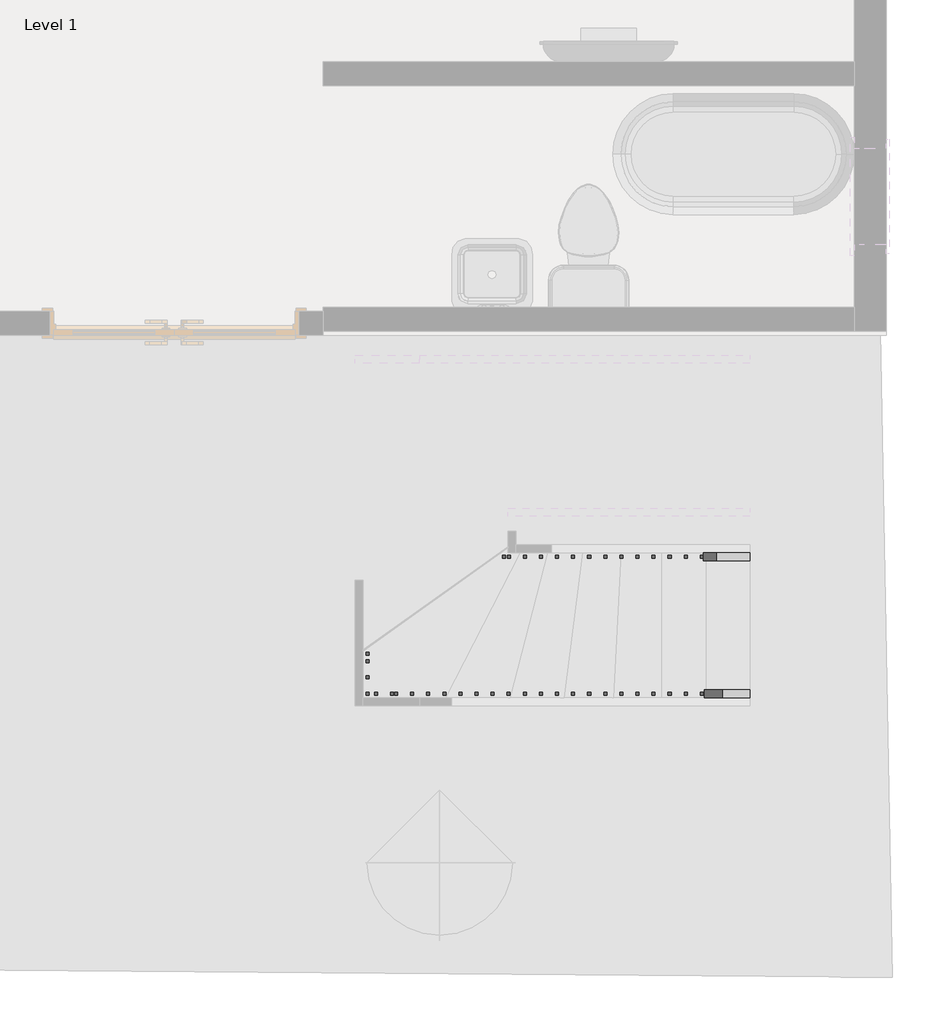
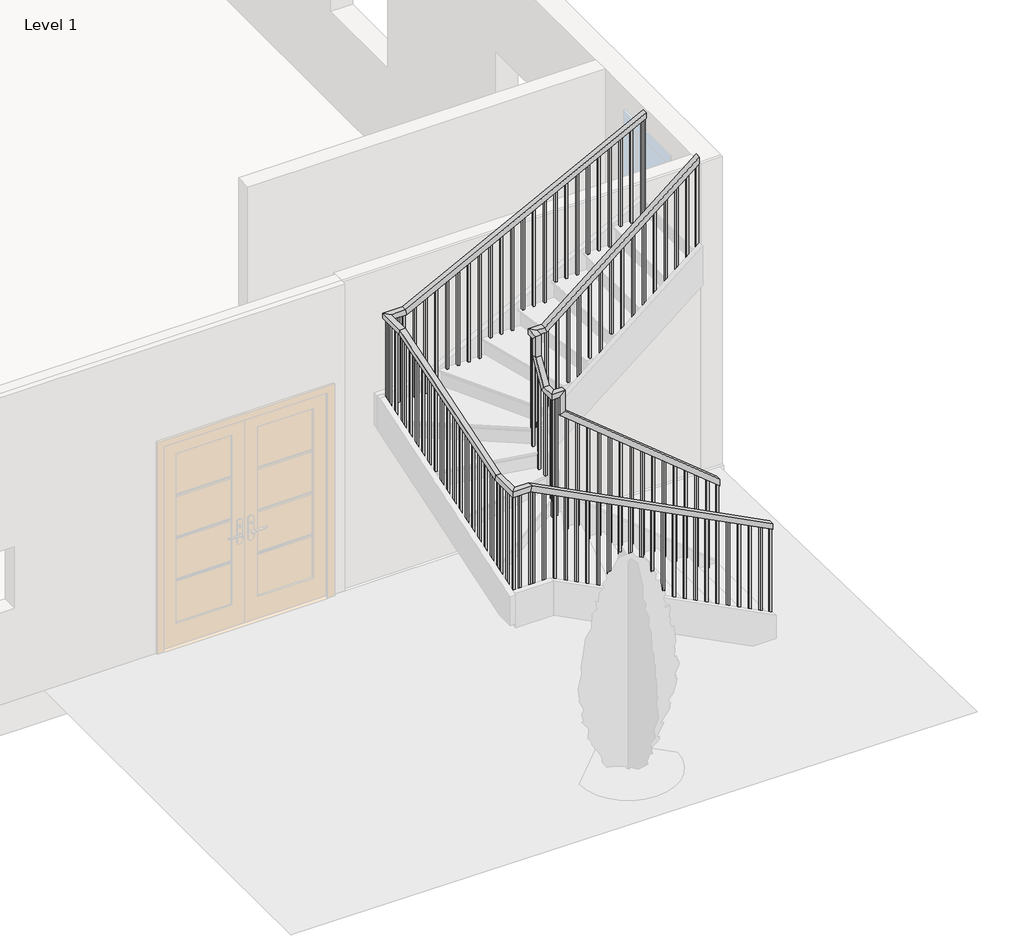
# One storey, part 2 of 3: 2 railings.
"""IFC4 building model written with IfcOpenShell, lengths in millimetres."""

from ifc_helpers import new_model, si_unit, frame, origin, place, context, project, spatial, polyline, outline, extrude, faceted_brep, element, save

model = new_model("IFC4")

# Units and contexts
model_context = context("Model", 3, world=origin())
ifc_project = project(units=[si_unit("LENGTHUNIT", "METRE", prefix="MILLI")], contexts=[model_context])

# Site, building, storey
site = spatial("IfcSite", under=ifc_project)
building = spatial("IfcBuilding", under=site)
storey = spatial("IfcBuildingStorey", under=building, Name="Level 1", Elevation=0.0)

# Railings
placement = place(None, origin())
element("IfcRailing", 1, ObjectType="Handrail - Rectangular", at=placement, inside=storey, context=model_context, shape_type="SolidModel", body=[
    faceted_brep([(-3425.4930658, -1530.446371, 1025.2529681), (-3425.4930658, -1530.446371, 959.7067088), (-3425.4930658, -1479.646371, 959.7067088), (-3425.4930658, -1479.646371, 1025.2529681), (-4877.0247577, -1530.446371, 2208.7848338), (-4927.8247577, -1530.446371, 2184.659247), (-4927.8247577, -1479.646371, 2184.659247), (-4877.0247577, -1479.646371, 2208.7848338), (-4877.0247577, -1530.446371, 2414.6281882), (-4927.8247577, -1530.446371, 2363.8281882), (-4927.8247577, -1479.646371, 2363.8281882), (-4877.0247577, -1479.646371, 2414.6281882), (-5004.0247577, -1530.446371, 2414.6281882), (-5004.0247577, -1530.446371, 2363.8281882), (-4953.2247577, -1479.646371, 2363.8281882), (-4953.2247577, -1479.646371, 2414.6281882), (-5004.0247577, -1403.446371, 2414.6281882), (-5004.0247577, -1374.3250371, 2363.8281882), (-4953.2247577, -1374.3250371, 2363.8281882), (-4953.2247577, -1403.446371, 2414.6281882), (-5004.0247577, -1276.446371, 2631.5051451), (-5004.0247577, -1225.646371, 2617.7256424), (-4953.2247577, -1225.646371, 2617.7256424), (-4953.2247577, -1276.446371, 2631.5051451), (-5004.0247577, -1276.446371, 2837.3484995), (-5004.0247577, -1225.646371, 2786.5484995), (-4953.2247577, -1225.646371, 2786.5484995), (-4953.2247577, -1276.446371, 2837.3484995), (-5004.0247577, -1149.446371, 2837.3484995), (-5004.0247577, -1149.446371, 2786.5484995), (-4953.2247577, -1200.246371, 2786.5484995), (-4953.2247577, -1200.246371, 2837.3484995), (-4877.0247577, -1149.446371, 2837.3484995), (-4858.9393446, -1149.446371, 2786.5484995), (-4858.9393446, -1200.246371, 2786.5484995), (-4877.0247577, -1200.246371, 2837.3484995), (-3425.4930658, -1149.446371, 4020.8803652), (-3425.4930658, -1200.246371, 4020.8803652), (-3425.4930658, -1200.246371, 3955.3341059), (-3425.4930658, -1149.446371, 3955.3341059)], [[[0, 1, 2, 3]], [[1, 0, 4, 5]], [[2, 1, 5, 6]], [[3, 2, 6, 7]], [[0, 3, 7, 4]], [[5, 4, 8, 9]], [[6, 5, 9, 10]], [[7, 6, 10, 11]], [[4, 7, 11, 8]], [[9, 8, 12, 13]], [[10, 9, 13, 14]], [[11, 10, 14, 15]], [[8, 11, 15, 12]], [[13, 12, 16, 17]], [[14, 13, 17, 18]], [[15, 14, 18, 19]], [[12, 15, 19, 16]], [[17, 16, 20, 21]], [[18, 17, 21, 22]], [[19, 18, 22, 23]], [[16, 19, 23, 20]], [[21, 20, 24, 25]], [[22, 21, 25, 26]], [[23, 22, 26, 27]], [[20, 23, 27, 24]], [[25, 24, 28, 29]], [[26, 25, 29, 30]], [[27, 26, 30, 31]], [[24, 27, 31, 28]], [[29, 28, 32, 33]], [[30, 29, 33, 34]], [[31, 30, 34, 35]], [[28, 31, 35, 32]], [[36, 37, 38, 39]], [[33, 32, 36, 39]], [[34, 33, 39, 38]], [[35, 34, 38, 37]], [[32, 35, 37, 36]]]),
    extrude(outline(polyline([(3881.7558784, -3515.7324013), (3866.2231262, -3534.7824013), (2878.6666667, -3534.7824013), (2878.6666667, -3515.7324013), (3881.7558784, -3515.7324013)])), frame((0.0, -1184.371371, 0.0), z_axis=(0.0, 1.0, 0.0), x_axis=(0.0, 0.0, 1.0)), (0.0, 0.0, 1.0), 19.05),
    extrude(outline(polyline([(3798.9145334, -3617.3324013), (3783.3817813, -3636.3824013), (2878.6666667, -3636.3824013), (2878.6666667, -3617.3324013), (3798.9145334, -3617.3324013)])), frame((0.0, -1184.371371, 0.0), z_axis=(0.0, 1.0, 0.0), x_axis=(0.0, 0.0, 1.0)), (0.0, 0.0, 1.0), 19.05),
    extrude(outline(polyline([(3716.0731885, -3718.9324013), (3700.5404364, -3737.9824013), (2709.3333333, -3737.9824013), (2709.3333333, -3718.9324013), (3716.0731885, -3718.9324013)])), frame((0.0, -1184.371371, 0.0), z_axis=(0.0, 1.0, 0.0), x_axis=(0.0, 0.0, 1.0)), (0.0, 0.0, 1.0), 19.05),
    extrude(outline(polyline([(3633.2318436, -3820.5324013), (3617.6990914, -3839.5824013), (2709.3333333, -3839.5824013), (2709.3333333, -3820.5324013), (3633.2318436, -3820.5324013)])), frame((0.0, -1184.371371, 0.0), z_axis=(0.0, 1.0, 0.0), x_axis=(0.0, 0.0, 1.0)), (0.0, 0.0, 1.0), 19.05),
    extrude(outline(polyline([(3550.3904987, -3922.1324013), (3534.8577465, -3941.1824013), (2709.3333333, -3941.1824013), (2709.3333333, -3922.1324013), (3550.3904987, -3922.1324013)])), frame((0.0, -1184.371371, 0.0), z_axis=(0.0, 1.0, 0.0), x_axis=(0.0, 0.0, 1.0)), (0.0, 0.0, 1.0), 19.05),
    extrude(outline(polyline([(3467.5491538, -4023.7324013), (3452.0164016, -4042.7824013), (2540.0, -4042.7824013), (2540.0, -4023.7324013), (3467.5491538, -4023.7324013)])), frame((0.0, -1184.371371, 0.0), z_axis=(0.0, 1.0, 0.0), x_axis=(0.0, 0.0, 1.0)), (0.0, 0.0, 1.0), 19.05),
    extrude(outline(polyline([(3384.7078088, -4125.3324013), (3369.1750567, -4144.3824013), (2540.0, -4144.3824013), (2540.0, -4125.3324013), (3384.7078088, -4125.3324013)])), frame((0.0, -1184.371371, 0.0), z_axis=(0.0, 1.0, 0.0), x_axis=(0.0, 0.0, 1.0)), (0.0, 0.0, 1.0), 19.05),
    extrude(outline(polyline([(3301.8664639, -4226.9324013), (3286.3337117, -4245.9824013), (2540.0, -4245.9824013), (2540.0, -4226.9324013), (3301.8664639, -4226.9324013)])), frame((0.0, -1184.371371, 0.0), z_axis=(0.0, 1.0, 0.0), x_axis=(0.0, 0.0, 1.0)), (0.0, 0.0, 1.0), 19.05),
    extrude(outline(polyline([(3219.025119, -4328.5324013), (3203.4923668, -4347.5824013), (2370.6666667, -4347.5824013), (2370.6666667, -4328.5324013), (3219.025119, -4328.5324013)])), frame((0.0, -1184.371371, 0.0), z_axis=(0.0, 1.0, 0.0), x_axis=(0.0, 0.0, 1.0)), (0.0, 0.0, 1.0), 19.05),
    extrude(outline(polyline([(3136.1837741, -4430.1324013), (3120.6510219, -4449.1824013), (2370.6666667, -4449.1824013), (2370.6666667, -4430.1324013), (3136.1837741, -4430.1324013)])), frame((0.0, -1184.371371, 0.0), z_axis=(0.0, 1.0, 0.0), x_axis=(0.0, 0.0, 1.0)), (0.0, 0.0, 1.0), 19.05),
    extrude(outline(polyline([(3053.3424291, -4531.7324013), (3037.809677, -4550.7824013), (2201.3333333, -4550.7824013), (2201.3333333, -4531.7324013), (3053.3424291, -4531.7324013)])), frame((0.0, -1184.371371, 0.0), z_axis=(0.0, 1.0, 0.0), x_axis=(0.0, 0.0, 1.0)), (0.0, 0.0, 1.0), 19.05),
    extrude(outline(polyline([(2970.5010842, -4633.3324013), (2954.9683321, -4652.3824013), (2201.3333333, -4652.3824013), (2201.3333333, -4633.3324013), (2970.5010842, -4633.3324013)])), frame((0.0, -1184.371371, 0.0), z_axis=(0.0, 1.0, 0.0), x_axis=(0.0, 0.0, 1.0)), (0.0, 0.0, 1.0), 19.05),
    extrude(outline(polyline([(2887.6597393, -4734.9324013), (2872.1269871, -4753.9824013), (2032.0, -4753.9824013), (2032.0, -4734.9324013), (2887.6597393, -4734.9324013)])), frame((0.0, -1184.371371, 0.0), z_axis=(0.0, 1.0, 0.0), x_axis=(0.0, 0.0, 1.0)), (0.0, 0.0, 1.0), 19.05),
    extrude(outline(polyline([(2804.8183944, -4836.5324013), (2789.2856422, -4855.5824013), (2032.0, -4855.5824013), (2032.0, -4836.5324013), (2804.8183944, -4836.5324013)])), frame((0.0, -1184.371371, 0.0), z_axis=(0.0, 1.0, 0.0), x_axis=(0.0, 0.0, 1.0)), (0.0, 0.0, 1.0), 19.05),
    extrude(outline(polyline([(-1296.5854672, 2496.5834745), (-1277.5354672, 2529.115018), (-1277.5354672, 1524.0), (-1296.5854672, 1524.0), (-1296.5854672, 2496.5834745)])), frame((-4988.1497577, 0.0, 0.0), z_axis=(1.0, 0.0, 0.0), x_axis=(0.0, 1.0, 0.0)), (0.0, 0.0, 1.0), 19.05),
    extrude(outline(polyline([(-1398.1854672, 2323.0819089), (-1379.1354672, 2355.6134525), (-1379.1354672, 1524.0), (-1398.1854672, 1524.0), (-1398.1854672, 2323.0819089)])), frame((-4988.1497577, 0.0, 0.0), z_axis=(1.0, 0.0, 0.0), x_axis=(0.0, 1.0, 0.0)), (0.0, 0.0, 1.0), 19.05),
    extrude(outline(polyline([(2111.7191617, -4838.3680658), (2127.2519138, -4857.4180658), (1016.0, -4857.4180658), (1016.0, -4838.3680658), (2111.7191617, -4838.3680658)])), frame((0.0, -1514.571371, 0.0), z_axis=(0.0, 1.0, 0.0), x_axis=(0.0, 0.0, 1.0)), (0.0, 0.0, 1.0), 19.05),
    extrude(outline(polyline([(2028.8778167, -4736.7680658), (2044.4105689, -4755.8180658), (1016.0, -4755.8180658), (1016.0, -4736.7680658), (2028.8778167, -4736.7680658)])), frame((0.0, -1514.571371, 0.0), z_axis=(0.0, 1.0, 0.0), x_axis=(0.0, 0.0, 1.0)), (0.0, 0.0, 1.0), 19.05),
    extrude(outline(polyline([(1946.0364718, -4635.1680658), (1961.569224, -4654.2180658), (846.6666667, -4654.2180658), (846.6666667, -4635.1680658), (1946.0364718, -4635.1680658)])), frame((0.0, -1514.571371, 0.0), z_axis=(0.0, 1.0, 0.0), x_axis=(0.0, 0.0, 1.0)), (0.0, 0.0, 1.0), 19.05),
    extrude(outline(polyline([(1863.1951269, -4533.5680658), (1878.7278791, -4552.6180658), (846.6666667, -4552.6180658), (846.6666667, -4533.5680658), (1863.1951269, -4533.5680658)])), frame((0.0, -1514.571371, 0.0), z_axis=(0.0, 1.0, 0.0), x_axis=(0.0, 0.0, 1.0)), (0.0, 0.0, 1.0), 19.05),
    extrude(outline(polyline([(1780.353782, -4431.9680658), (1795.8865341, -4451.0180658), (677.3333333, -4451.0180658), (677.3333333, -4431.9680658), (1780.353782, -4431.9680658)])), frame((0.0, -1514.571371, 0.0), z_axis=(0.0, 1.0, 0.0), x_axis=(0.0, 0.0, 1.0)), (0.0, 0.0, 1.0), 19.05),
    extrude(outline(polyline([(1697.5124371, -4330.3680658), (1713.0451892, -4349.4180658), (677.3333333, -4349.4180658), (677.3333333, -4330.3680658), (1697.5124371, -4330.3680658)])), frame((0.0, -1514.571371, 0.0), z_axis=(0.0, 1.0, 0.0), x_axis=(0.0, 0.0, 1.0)), (0.0, 0.0, 1.0), 19.05),
    extrude(outline(polyline([(1614.6710921, -4228.7680658), (1630.2038443, -4247.8180658), (508.0, -4247.8180658), (508.0, -4228.7680658), (1614.6710921, -4228.7680658)])), frame((0.0, -1514.571371, 0.0), z_axis=(0.0, 1.0, 0.0), x_axis=(0.0, 0.0, 1.0)), (0.0, 0.0, 1.0), 19.05),
    extrude(outline(polyline([(1531.8297472, -4127.1680658), (1547.3624994, -4146.2180658), (508.0, -4146.2180658), (508.0, -4127.1680658), (1531.8297472, -4127.1680658)])), frame((0.0, -1514.571371, 0.0), z_axis=(0.0, 1.0, 0.0), x_axis=(0.0, 0.0, 1.0)), (0.0, 0.0, 1.0), 19.05),
    extrude(outline(polyline([(1448.9884023, -4025.5680658), (1464.5211545, -4044.6180658), (508.0, -4044.6180658), (508.0, -4025.5680658), (1448.9884023, -4025.5680658)])), frame((0.0, -1514.571371, 0.0), z_axis=(0.0, 1.0, 0.0), x_axis=(0.0, 0.0, 1.0)), (0.0, 0.0, 1.0), 19.05),
    extrude(outline(polyline([(1366.1470574, -3923.9680658), (1381.6798095, -3943.0180658), (338.6666667, -3943.0180658), (338.6666667, -3923.9680658), (1366.1470574, -3923.9680658)])), frame((0.0, -1514.571371, 0.0), z_axis=(0.0, 1.0, 0.0), x_axis=(0.0, 0.0, 1.0)), (0.0, 0.0, 1.0), 19.05),
    extrude(outline(polyline([(1283.3057124, -3822.3680658), (1298.8384646, -3841.4180658), (338.6666667, -3841.4180658), (338.6666667, -3822.3680658), (1283.3057124, -3822.3680658)])), frame((0.0, -1514.571371, 0.0), z_axis=(0.0, 1.0, 0.0), x_axis=(0.0, 0.0, 1.0)), (0.0, 0.0, 1.0), 19.05),
    extrude(outline(polyline([(1200.4643675, -3720.7680658), (1215.9971197, -3739.8180658), (338.6666667, -3739.8180658), (338.6666667, -3720.7680658), (1200.4643675, -3720.7680658)])), frame((0.0, -1514.571371, 0.0), z_axis=(0.0, 1.0, 0.0), x_axis=(0.0, 0.0, 1.0)), (0.0, 0.0, 1.0), 19.05),
    extrude(outline(polyline([(1117.6230226, -3619.1680658), (1133.1557748, -3638.2180658), (169.3333333, -3638.2180658), (169.3333333, -3619.1680658), (1117.6230226, -3619.1680658)])), frame((0.0, -1514.571371, 0.0), z_axis=(0.0, 1.0, 0.0), x_axis=(0.0, 0.0, 1.0)), (0.0, 0.0, 1.0), 19.05),
    extrude(outline(polyline([(1034.7816777, -3517.5680658), (1050.3144298, -3536.6180658), (169.3333333, -3536.6180658), (169.3333333, -3517.5680658), (1034.7816777, -3517.5680658)])), frame((0.0, -1514.571371, 0.0), z_axis=(0.0, 1.0, 0.0), x_axis=(0.0, 0.0, 1.0)), (0.0, 0.0, 1.0), 19.05),
    extrude(outline(polyline([(-4957.1824013, -1184.371371), (-4957.1824013, -1165.321371), (-4938.1324013, -1165.321371), (-4938.1324013, -1184.371371), (-4957.1824013, -1184.371371)])), frame((0.0, 0.0, 1862.6666667), z_axis=(0.0, 0.0, 1.0), x_axis=(1.0, 0.0, 0.0)), (0.0, 0.0, 1.0), 923.8818329),
    extrude(outline(polyline([(-4969.0997577, -1184.371371), (-4988.1497577, -1184.371371), (-4988.1497577, -1165.321371), (-4969.0997577, -1165.321371), (-4969.0997577, -1184.371371)])), frame((0.0, 0.0, 1862.6666667), z_axis=(0.0, 0.0, 1.0), x_axis=(1.0, 0.0, 0.0)), (0.0, 0.0, 1.0), 923.8818329),
    extrude(outline(polyline([(-4969.0997577, -1199.1572747), (-4988.1497577, -1199.1572747), (-4988.1497577, -1180.1072747), (-4969.0997577, -1180.1072747), (-4969.0997577, -1199.1572747)])), frame((0.0, 0.0, 1693.3333333), z_axis=(0.0, 0.0, 1.0), x_axis=(1.0, 0.0, 0.0)), (0.0, 0.0, 1.0), 1093.2151662),
    extrude(outline(polyline([(-4969.0997577, -1499.7854672), (-4988.1497577, -1499.7854672), (-4988.1497577, -1480.7354672), (-4969.0997577, -1480.7354672), (-4969.0997577, -1499.7854672)])), frame((0.0, 0.0, 1354.6666667), z_axis=(0.0, 0.0, 1.0), x_axis=(1.0, 0.0, 0.0)), (0.0, 0.0, 1.0), 1009.1615215),
    extrude(outline(polyline([(-4969.0997577, -1495.521371), (-4969.0997577, -1514.571371), (-4988.1497577, -1514.571371), (-4988.1497577, -1495.521371), (-4969.0997577, -1495.521371)])), frame((0.0, 0.0, 1185.3333333), z_axis=(0.0, 0.0, 1.0), x_axis=(1.0, 0.0, 0.0)), (0.0, 0.0, 1.0), 1178.4948549),
    extrude(outline(polyline([(-4938.1324013, -1495.521371), (-4938.1324013, -1514.571371), (-4957.1824013, -1514.571371), (-4957.1824013, -1495.521371), (-4938.1324013, -1495.521371)])), frame((0.0, 0.0, 1185.3333333), z_axis=(0.0, 0.0, 1.0), x_axis=(1.0, 0.0, 0.0)), (0.0, 0.0, 1.0), 1178.4948549),
    extrude(outline(polyline([(3955.3341059, -3425.4930658), (3939.8013537, -3444.5430658), (2878.6666667, -3444.5430658), (2878.6666667, -3425.4930658), (3955.3341059, -3425.4930658)])), frame((0.0, -1184.371371, 0.0), z_axis=(0.0, 1.0, 0.0), x_axis=(0.0, 0.0, 1.0)), (0.0, 0.0, 1.0), 19.05),
    extrude(outline(polyline([(959.7067088, -3425.4930658), (975.239461, -3444.5430658), (169.3333333, -3444.5430658), (169.3333333, -3425.4930658), (959.7067088, -3425.4930658)])), frame((0.0, -1514.571371, 0.0), z_axis=(0.0, 1.0, 0.0), x_axis=(0.0, 0.0, 1.0)), (0.0, 0.0, 1.0), 19.05),
])
element("IfcRailing", 2, ObjectType="Handrail - Rectangular", at=placement, inside=storey, context=model_context, shape_type="SolidModel", body=[
    faceted_brep([(-3425.4930658, -2394.046371, 1109.0771751), (-3425.4930658, -2394.046371, 1051.9280057), (-3425.4930658, -2343.246371, 1051.9280057), (-3425.4930658, -2343.246371, 1109.0771751), (-5685.4749223, -2394.046371, 2273.7644996), (-5697.7949736, -2394.046371, 2222.9644996), (-5697.7949736, -2343.246371, 2222.9644996), (-5685.4749223, -2343.246371, 2273.7644996), (-5867.6247577, -2394.046371, 2273.7644996), (-5867.6247577, -2394.046371, 2222.9644996), (-5816.8247577, -2343.246371, 2222.9644996), (-5816.8247577, -2343.246371, 2273.7644996), (-5867.6247577, -2116.8924184, 2273.7644996), (-5867.6247577, -2108.9418422, 2222.9644996), (-5816.8247577, -2108.9418422, 2222.9644996), (-5816.8247577, -2116.8924184, 2273.7644996), (-5867.6247577, -563.0003236, 2772.3688337), (-5867.6247577, -555.0497475, 2721.5688337), (-5816.8247577, -555.0497475, 2721.5688337), (-5816.8247577, -563.0003236, 2772.3688337), (-5867.6247577, -285.846371, 2772.3688337), (-5867.6247577, -285.846371, 2721.5688337), (-5816.8247577, -336.646371, 2721.5688337), (-5816.8247577, -336.646371, 2772.3688337), (-5685.4749223, -285.846371, 2772.3688337), (-5673.154871, -285.846371, 2721.5688337), (-5673.154871, -336.646371, 2721.5688337), (-5685.4749223, -336.646371, 2772.3688337), (-3425.4930658, -285.846371, 3937.0561582), (-3425.4930658, -336.646371, 3937.0561582), (-3425.4930658, -336.646371, 3879.9069889), (-3425.4930658, -285.846371, 3879.9069889)], [[[0, 1, 2, 3]], [[1, 0, 4, 5]], [[2, 1, 5, 6]], [[3, 2, 6, 7]], [[0, 3, 7, 4]], [[5, 4, 8, 9]], [[6, 5, 9, 10]], [[7, 6, 10, 11]], [[4, 7, 11, 8]], [[9, 8, 12, 13]], [[10, 9, 13, 14]], [[11, 10, 14, 15]], [[8, 11, 15, 12]], [[13, 12, 16, 17]], [[14, 13, 17, 18]], [[15, 14, 18, 19]], [[12, 15, 19, 16]], [[17, 16, 20, 21]], [[18, 17, 21, 22]], [[19, 18, 22, 23]], [[16, 19, 23, 20]], [[21, 20, 24, 25]], [[22, 21, 25, 26]], [[23, 22, 26, 27]], [[20, 23, 27, 24]], [[28, 29, 30, 31]], [[25, 24, 28, 31]], [[26, 25, 31, 30]], [[27, 26, 30, 29]], [[24, 27, 29, 28]]]),
    extrude(outline(polyline([(3862.2268642, -3459.7999223), (2878.6666667, -3459.7999223), (2878.6666667, -3440.7499223), (3872.0443296, -3440.7499223), (3862.2268642, -3459.7999223)])), frame((0.0, -320.771371, 0.0), z_axis=(0.0, 1.0, 0.0), x_axis=(0.0, 0.0, 1.0)), (0.0, 0.0, 1.0), 19.05),
    extrude(outline(polyline([(3809.8670491, -3561.3999223), (2878.6666667, -3561.3999223), (2878.6666667, -3542.3499223), (3819.6845145, -3542.3499223), (3809.8670491, -3561.3999223)])), frame((0.0, -320.771371, 0.0), z_axis=(0.0, 1.0, 0.0), x_axis=(0.0, 0.0, 1.0)), (0.0, 0.0, 1.0), 19.05),
    extrude(outline(polyline([(3757.507234, -3662.9999223), (2878.6666667, -3662.9999223), (2878.6666667, -3643.9499223), (3767.3246993, -3643.9499223), (3757.507234, -3662.9999223)])), frame((0.0, -320.771371, 0.0), z_axis=(0.0, 1.0, 0.0), x_axis=(0.0, 0.0, 1.0)), (0.0, 0.0, 1.0), 19.05),
    extrude(outline(polyline([(3705.1474189, -3764.5999223), (2709.3333333, -3764.5999223), (2709.3333333, -3745.5499223), (3714.9648842, -3745.5499223), (3705.1474189, -3764.5999223)])), frame((0.0, -320.771371, 0.0), z_axis=(0.0, 1.0, 0.0), x_axis=(0.0, 0.0, 1.0)), (0.0, 0.0, 1.0), 19.05),
    extrude(outline(polyline([(3652.7876038, -3866.1999223), (2709.3333333, -3866.1999223), (2709.3333333, -3847.1499223), (3662.6050691, -3847.1499223), (3652.7876038, -3866.1999223)])), frame((0.0, -320.771371, 0.0), z_axis=(0.0, 1.0, 0.0), x_axis=(0.0, 0.0, 1.0)), (0.0, 0.0, 1.0), 19.05),
    extrude(outline(polyline([(3600.4277887, -3967.7999223), (2709.3333333, -3967.7999223), (2709.3333333, -3948.7499223), (3610.245254, -3948.7499223), (3600.4277887, -3967.7999223)])), frame((0.0, -320.771371, 0.0), z_axis=(0.0, 1.0, 0.0), x_axis=(0.0, 0.0, 1.0)), (0.0, 0.0, 1.0), 19.05),
    extrude(outline(polyline([(3548.0679735, -4069.3999223), (2540.0, -4069.3999223), (2540.0, -4050.3499223), (3557.8854389, -4050.3499223), (3548.0679735, -4069.3999223)])), frame((0.0, -320.771371, 0.0), z_axis=(0.0, 1.0, 0.0), x_axis=(0.0, 0.0, 1.0)), (0.0, 0.0, 1.0), 19.05),
    extrude(outline(polyline([(3495.7081584, -4170.9999223), (2540.0, -4170.9999223), (2540.0, -4151.9499223), (3505.5256238, -4151.9499223), (3495.7081584, -4170.9999223)])), frame((0.0, -320.771371, 0.0), z_axis=(0.0, 1.0, 0.0), x_axis=(0.0, 0.0, 1.0)), (0.0, 0.0, 1.0), 19.05),
    extrude(outline(polyline([(3443.3483433, -4272.5999223), (2540.0, -4272.5999223), (2540.0, -4253.5499223), (3453.1658086, -4253.5499223), (3443.3483433, -4272.5999223)])), frame((0.0, -320.771371, 0.0), z_axis=(0.0, 1.0, 0.0), x_axis=(0.0, 0.0, 1.0)), (0.0, 0.0, 1.0), 19.05),
    extrude(outline(polyline([(3390.9885282, -4374.1999223), (2370.6666667, -4374.1999223), (2370.6666667, -4355.1499223), (3400.8059935, -4355.1499223), (3390.9885282, -4374.1999223)])), frame((0.0, -320.771371, 0.0), z_axis=(0.0, 1.0, 0.0), x_axis=(0.0, 0.0, 1.0)), (0.0, 0.0, 1.0), 19.05),
    extrude(outline(polyline([(3338.6287131, -4475.7999223), (2370.6666667, -4475.7999223), (2370.6666667, -4456.7499223), (3348.4461784, -4456.7499223), (3338.6287131, -4475.7999223)])), frame((0.0, -320.771371, 0.0), z_axis=(0.0, 1.0, 0.0), x_axis=(0.0, 0.0, 1.0)), (0.0, 0.0, 1.0), 19.05),
    extrude(outline(polyline([(3286.268898, -4577.3999223), (2370.6666667, -4577.3999223), (2370.6666667, -4558.3499223), (3296.0863633, -4558.3499223), (3286.268898, -4577.3999223)])), frame((0.0, -320.771371, 0.0), z_axis=(0.0, 1.0, 0.0), x_axis=(0.0, 0.0, 1.0)), (0.0, 0.0, 1.0), 19.05),
    extrude(outline(polyline([(3233.9090828, -4678.9999223), (2201.3333333, -4678.9999223), (2201.3333333, -4659.9499223), (3243.7265482, -4659.9499223), (3233.9090828, -4678.9999223)])), frame((0.0, -320.771371, 0.0), z_axis=(0.0, 1.0, 0.0), x_axis=(0.0, 0.0, 1.0)), (0.0, 0.0, 1.0), 19.05),
    extrude(outline(polyline([(3181.5492677, -4780.5999223), (2201.3333333, -4780.5999223), (2201.3333333, -4761.5499223), (3191.3667331, -4761.5499223), (3181.5492677, -4780.5999223)])), frame((0.0, -320.771371, 0.0), z_axis=(0.0, 1.0, 0.0), x_axis=(0.0, 0.0, 1.0)), (0.0, 0.0, 1.0), 19.05),
    extrude(outline(polyline([(3129.1894526, -4882.1999223), (2201.3333333, -4882.1999223), (2201.3333333, -4863.1499223), (3139.0069179, -4863.1499223), (3129.1894526, -4882.1999223)])), frame((0.0, -320.771371, 0.0), z_axis=(0.0, 1.0, 0.0), x_axis=(0.0, 0.0, 1.0)), (0.0, 0.0, 1.0), 19.05),
    extrude(outline(polyline([(3076.8296375, -4983.7999223), (2032.0, -4983.7999223), (2032.0, -4964.7499223), (3086.6471028, -4964.7499223), (3076.8296375, -4983.7999223)])), frame((0.0, -320.771371, 0.0), z_axis=(0.0, 1.0, 0.0), x_axis=(0.0, 0.0, 1.0)), (0.0, 0.0, 1.0), 19.05),
    extrude(outline(polyline([(3024.4698224, -5085.3999223), (2032.0, -5085.3999223), (2032.0, -5066.3499223), (3034.2872877, -5066.3499223), (3024.4698224, -5085.3999223)])), frame((0.0, -320.771371, 0.0), z_axis=(0.0, 1.0, 0.0), x_axis=(0.0, 0.0, 1.0)), (0.0, 0.0, 1.0), 19.05),
    extrude(outline(polyline([(2972.1100073, -5186.9999223), (2032.0, -5186.9999223), (2032.0, -5167.9499223), (2981.9274726, -5167.9499223), (2972.1100073, -5186.9999223)])), frame((0.0, -320.771371, 0.0), z_axis=(0.0, 1.0, 0.0), x_axis=(0.0, 0.0, 1.0)), (0.0, 0.0, 1.0), 19.05),
    extrude(outline(polyline([(2919.7501921, -5288.5999223), (2032.0, -5288.5999223), (2032.0, -5269.5499223), (2929.5676575, -5269.5499223), (2919.7501921, -5288.5999223)])), frame((0.0, -320.771371, 0.0), z_axis=(0.0, 1.0, 0.0), x_axis=(0.0, 0.0, 1.0)), (0.0, 0.0, 1.0), 19.05),
    extrude(outline(polyline([(2867.390377, -5390.1999223), (1862.6666667, -5390.1999223), (1862.6666667, -5371.1499223), (2877.2078424, -5371.1499223), (2867.390377, -5390.1999223)])), frame((0.0, -320.771371, 0.0), z_axis=(0.0, 1.0, 0.0), x_axis=(0.0, 0.0, 1.0)), (0.0, 0.0, 1.0), 19.05),
    extrude(outline(polyline([(2815.0305619, -5491.7999223), (1862.6666667, -5491.7999223), (1862.6666667, -5472.7499223), (2824.8480272, -5472.7499223), (2815.0305619, -5491.7999223)])), frame((0.0, -320.771371, 0.0), z_axis=(0.0, 1.0, 0.0), x_axis=(0.0, 0.0, 1.0)), (0.0, 0.0, 1.0), 19.05),
    extrude(outline(polyline([(2762.6707468, -5593.3999223), (1862.6666667, -5593.3999223), (1862.6666667, -5574.3499223), (2772.4882121, -5574.3499223), (2762.6707468, -5593.3999223)])), frame((0.0, -320.771371, 0.0), z_axis=(0.0, 1.0, 0.0), x_axis=(0.0, 0.0, 1.0)), (0.0, 0.0, 1.0), 19.05),
    extrude(outline(polyline([(-5750.1497577, -301.721371), (-5731.0997577, -301.721371), (-5731.0997577, -320.771371), (-5750.1497577, -320.771371), (-5750.1497577, -301.721371)])), frame((0.0, 0.0, 1862.6666667), z_axis=(0.0, 0.0, 1.0), x_axis=(1.0, 0.0, 0.0)), (0.0, 0.0, 1.0), 858.902167),
    extrude(outline(polyline([(-5851.7497577, -369.3253236), (-5851.7497577, -350.2753236), (-5832.6997577, -350.2753236), (-5832.6997577, -369.3253236), (-5851.7497577, -369.3253236)])), frame((0.0, 0.0, 1862.6666667), z_axis=(0.0, 0.0, 1.0), x_axis=(1.0, 0.0, 0.0)), (0.0, 0.0, 1.0), 858.902167),
    extrude(outline(polyline([(-5851.7497577, -470.9253236), (-5851.7497577, -451.8753236), (-5832.6997577, -451.8753236), (-5832.6997577, -470.9253236), (-5851.7497577, -470.9253236)])), frame((0.0, 0.0, 1862.6666667), z_axis=(0.0, 0.0, 1.0), x_axis=(1.0, 0.0, 0.0)), (0.0, 0.0, 1.0), 858.902167),
    extrude(outline(polyline([(-583.3674184, 2712.4824155), (-583.3674184, 1693.3333333), (-602.4174184, 1693.3333333), (-602.4174184, 2706.3697564), (-583.3674184, 2712.4824155)])), frame((-5851.7497577, 0.0, 0.0), z_axis=(1.0, 0.0, 0.0), x_axis=(0.0, 1.0, 0.0)), (0.0, 0.0, 1.0), 19.05),
    extrude(outline(polyline([(-684.9674184, 2679.8815673), (-684.9674184, 1693.3333333), (-704.0174184, 1693.3333333), (-704.0174184, 2673.7689082), (-684.9674184, 2679.8815673)])), frame((-5851.7497577, 0.0, 0.0), z_axis=(1.0, 0.0, 0.0), x_axis=(0.0, 1.0, 0.0)), (0.0, 0.0, 1.0), 19.05),
    extrude(outline(polyline([(-786.5674184, 2647.280719), (-786.5674184, 1693.3333333), (-805.6174184, 1693.3333333), (-805.6174184, 2641.16806), (-786.5674184, 2647.280719)])), frame((-5851.7497577, 0.0, 0.0), z_axis=(1.0, 0.0, 0.0), x_axis=(0.0, 1.0, 0.0)), (0.0, 0.0, 1.0), 19.05),
    extrude(outline(polyline([(-888.1674184, 2614.6798708), (-888.1674184, 1693.3333333), (-907.2174184, 1693.3333333), (-907.2174184, 2608.5672118), (-888.1674184, 2614.6798708)])), frame((-5851.7497577, 0.0, 0.0), z_axis=(1.0, 0.0, 0.0), x_axis=(0.0, 1.0, 0.0)), (0.0, 0.0, 1.0), 19.05),
    extrude(outline(polyline([(-989.7674184, 2582.0790226), (-989.7674184, 1693.3333333), (-1008.8174184, 1693.3333333), (-1008.8174184, 2575.9663635), (-989.7674184, 2582.0790226)])), frame((-5851.7497577, 0.0, 0.0), z_axis=(1.0, 0.0, 0.0), x_axis=(0.0, 1.0, 0.0)), (0.0, 0.0, 1.0), 19.05),
    extrude(outline(polyline([(-1091.3674184, 2549.4781744), (-1091.3674184, 1693.3333333), (-1110.4174184, 1693.3333333), (-1110.4174184, 2543.3655153), (-1091.3674184, 2549.4781744)])), frame((-5851.7497577, 0.0, 0.0), z_axis=(1.0, 0.0, 0.0), x_axis=(0.0, 1.0, 0.0)), (0.0, 0.0, 1.0), 19.05),
    extrude(outline(polyline([(-1192.9674184, 2516.8773261), (-1192.9674184, 1524.0), (-1212.0174184, 1524.0), (-1212.0174184, 2510.7646671), (-1192.9674184, 2516.8773261)])), frame((-5851.7497577, 0.0, 0.0), z_axis=(1.0, 0.0, 0.0), x_axis=(0.0, 1.0, 0.0)), (0.0, 0.0, 1.0), 19.05),
    extrude(outline(polyline([(-1294.5674184, 2484.2764779), (-1294.5674184, 1524.0), (-1313.6174184, 1524.0), (-1313.6174184, 2478.1638189), (-1294.5674184, 2484.2764779)])), frame((-5851.7497577, 0.0, 0.0), z_axis=(1.0, 0.0, 0.0), x_axis=(0.0, 1.0, 0.0)), (0.0, 0.0, 1.0), 19.05),
    extrude(outline(polyline([(-1396.1674184, 2451.6756297), (-1396.1674184, 1524.0), (-1415.2174184, 1524.0), (-1415.2174184, 2445.5629706), (-1396.1674184, 2451.6756297)])), frame((-5851.7497577, 0.0, 0.0), z_axis=(1.0, 0.0, 0.0), x_axis=(0.0, 1.0, 0.0)), (0.0, 0.0, 1.0), 19.05),
    extrude(outline(polyline([(-1497.7674184, 2419.0747814), (-1497.7674184, 1524.0), (-1516.8174184, 1524.0), (-1516.8174184, 2412.9621224), (-1497.7674184, 2419.0747814)])), frame((-5851.7497577, 0.0, 0.0), z_axis=(1.0, 0.0, 0.0), x_axis=(0.0, 1.0, 0.0)), (0.0, 0.0, 1.0), 19.05),
    extrude(outline(polyline([(-1599.3674184, 2386.4739332), (-1599.3674184, 1354.6666667), (-1618.4174184, 1354.6666667), (-1618.4174184, 2380.3612742), (-1599.3674184, 2386.4739332)])), frame((-5851.7497577, 0.0, 0.0), z_axis=(1.0, 0.0, 0.0), x_axis=(0.0, 1.0, 0.0)), (0.0, 0.0, 1.0), 19.05),
    extrude(outline(polyline([(-1700.9674184, 2353.873085), (-1700.9674184, 1354.6666667), (-1720.0174184, 1354.6666667), (-1720.0174184, 2347.7604259), (-1700.9674184, 2353.873085)])), frame((-5851.7497577, 0.0, 0.0), z_axis=(1.0, 0.0, 0.0), x_axis=(0.0, 1.0, 0.0)), (0.0, 0.0, 1.0), 19.05),
    extrude(outline(polyline([(-1802.5674184, 2321.2722368), (-1802.5674184, 1354.6666667), (-1821.6174184, 1354.6666667), (-1821.6174184, 2315.1595777), (-1802.5674184, 2321.2722368)])), frame((-5851.7497577, 0.0, 0.0), z_axis=(1.0, 0.0, 0.0), x_axis=(0.0, 1.0, 0.0)), (0.0, 0.0, 1.0), 19.05),
    extrude(outline(polyline([(-1904.1674184, 2288.6713885), (-1904.1674184, 1354.6666667), (-1923.2174184, 1354.6666667), (-1923.2174184, 2282.5587295), (-1904.1674184, 2288.6713885)])), frame((-5851.7497577, 0.0, 0.0), z_axis=(1.0, 0.0, 0.0), x_axis=(0.0, 1.0, 0.0)), (0.0, 0.0, 1.0), 19.05),
    extrude(outline(polyline([(-2005.7674184, 2256.0705403), (-2005.7674184, 1354.6666667), (-2024.8174184, 1354.6666667), (-2024.8174184, 2249.9578813), (-2005.7674184, 2256.0705403)])), frame((-5851.7497577, 0.0, 0.0), z_axis=(1.0, 0.0, 0.0), x_axis=(0.0, 1.0, 0.0)), (0.0, 0.0, 1.0), 19.05),
    extrude(outline(polyline([(-5851.7497577, -2174.971371), (-5851.7497577, -2155.921371), (-5832.6997577, -2155.921371), (-5832.6997577, -2174.971371), (-5851.7497577, -2174.971371)])), frame((0.0, 0.0, 1185.3333333), z_axis=(0.0, 0.0, 1.0), x_axis=(1.0, 0.0, 0.0)), (0.0, 0.0, 1.0), 1037.6311663),
    extrude(outline(polyline([(-5851.7497577, -2276.571371), (-5851.7497577, -2257.521371), (-5832.6997577, -2257.521371), (-5832.6997577, -2276.571371), (-5851.7497577, -2276.571371)])), frame((0.0, 0.0, 1185.3333333), z_axis=(0.0, 0.0, 1.0), x_axis=(1.0, 0.0, 0.0)), (0.0, 0.0, 1.0), 1037.6311663),
    extrude(outline(polyline([(-5777.5499223, -2378.171371), (-5796.5999223, -2378.171371), (-5796.5999223, -2359.121371), (-5777.5499223, -2359.121371), (-5777.5499223, -2378.171371)])), frame((0.0, 0.0, 1185.3333333), z_axis=(0.0, 0.0, 1.0), x_axis=(1.0, 0.0, 0.0)), (0.0, 0.0, 1.0), 1037.6311663),
    extrude(outline(polyline([(2208.752671, -5670.2180658), (1185.3333333, -5670.2180658), (1185.3333333, -5651.1680658), (2198.9352056, -5651.1680658), (2208.752671, -5670.2180658)])), frame((0.0, -2378.171371, 0.0), z_axis=(0.0, 1.0, 0.0), x_axis=(0.0, 0.0, 1.0)), (0.0, 0.0, 1.0), 19.05),
    extrude(outline(polyline([(2156.3928558, -5568.6180658), (1185.3333333, -5568.6180658), (1185.3333333, -5549.5680658), (2146.5753905, -5549.5680658), (2156.3928558, -5568.6180658)])), frame((0.0, -2378.171371, 0.0), z_axis=(0.0, 1.0, 0.0), x_axis=(0.0, 0.0, 1.0)), (0.0, 0.0, 1.0), 19.05),
    extrude(outline(polyline([(2104.0330407, -5467.0180658), (1185.3333333, -5467.0180658), (1185.3333333, -5447.9680658), (2094.2155754, -5447.9680658), (2104.0330407, -5467.0180658)])), frame((0.0, -2378.171371, 0.0), z_axis=(0.0, 1.0, 0.0), x_axis=(0.0, 0.0, 1.0)), (0.0, 0.0, 1.0), 19.05),
    extrude(outline(polyline([(2051.6732256, -5365.4180658), (1185.3333333, -5365.4180658), (1185.3333333, -5346.3680658), (2041.8557603, -5346.3680658), (2051.6732256, -5365.4180658)])), frame((0.0, -2378.171371, 0.0), z_axis=(0.0, 1.0, 0.0), x_axis=(0.0, 0.0, 1.0)), (0.0, 0.0, 1.0), 19.05),
    extrude(outline(polyline([(1999.3134105, -5263.8180658), (1016.0, -5263.8180658), (1016.0, -5244.7680658), (1989.4959452, -5244.7680658), (1999.3134105, -5263.8180658)])), frame((0.0, -2378.171371, 0.0), z_axis=(0.0, 1.0, 0.0), x_axis=(0.0, 0.0, 1.0)), (0.0, 0.0, 1.0), 19.05),
    extrude(outline(polyline([(1946.9535954, -5162.2180658), (1016.0, -5162.2180658), (1016.0, -5143.1680658), (1937.13613, -5143.1680658), (1946.9535954, -5162.2180658)])), frame((0.0, -2378.171371, 0.0), z_axis=(0.0, 1.0, 0.0), x_axis=(0.0, 0.0, 1.0)), (0.0, 0.0, 1.0), 19.05),
    extrude(outline(polyline([(1894.5937803, -5060.6180658), (1016.0, -5060.6180658), (1016.0, -5041.5680658), (1884.7763149, -5041.5680658), (1894.5937803, -5060.6180658)])), frame((0.0, -2378.171371, 0.0), z_axis=(0.0, 1.0, 0.0), x_axis=(0.0, 0.0, 1.0)), (0.0, 0.0, 1.0), 19.05),
    extrude(outline(polyline([(1842.2339651, -4959.0180658), (1016.0, -4959.0180658), (1016.0, -4939.9680658), (1832.4164998, -4939.9680658), (1842.2339651, -4959.0180658)])), frame((0.0, -2378.171371, 0.0), z_axis=(0.0, 1.0, 0.0), x_axis=(0.0, 0.0, 1.0)), (0.0, 0.0, 1.0), 19.05),
    extrude(outline(polyline([(1789.87415, -4857.4180658), (846.6666667, -4857.4180658), (846.6666667, -4838.3680658), (1780.0566847, -4838.3680658), (1789.87415, -4857.4180658)])), frame((0.0, -2378.171371, 0.0), z_axis=(0.0, 1.0, 0.0), x_axis=(0.0, 0.0, 1.0)), (0.0, 0.0, 1.0), 19.05),
    extrude(outline(polyline([(1737.5143349, -4755.8180658), (846.6666667, -4755.8180658), (846.6666667, -4736.7680658), (1727.6968696, -4736.7680658), (1737.5143349, -4755.8180658)])), frame((0.0, -2378.171371, 0.0), z_axis=(0.0, 1.0, 0.0), x_axis=(0.0, 0.0, 1.0)), (0.0, 0.0, 1.0), 19.05),
    extrude(outline(polyline([(1685.1545198, -4654.2180658), (846.6666667, -4654.2180658), (846.6666667, -4635.1680658), (1675.3370545, -4635.1680658), (1685.1545198, -4654.2180658)])), frame((0.0, -2378.171371, 0.0), z_axis=(0.0, 1.0, 0.0), x_axis=(0.0, 0.0, 1.0)), (0.0, 0.0, 1.0), 19.05),
    extrude(outline(polyline([(1632.7947047, -4552.6180658), (677.3333333, -4552.6180658), (677.3333333, -4533.5680658), (1622.9772393, -4533.5680658), (1632.7947047, -4552.6180658)])), frame((0.0, -2378.171371, 0.0), z_axis=(0.0, 1.0, 0.0), x_axis=(0.0, 0.0, 1.0)), (0.0, 0.0, 1.0), 19.05),
    extrude(outline(polyline([(1580.4348896, -4451.0180658), (677.3333333, -4451.0180658), (677.3333333, -4431.9680658), (1570.6174242, -4431.9680658), (1580.4348896, -4451.0180658)])), frame((0.0, -2378.171371, 0.0), z_axis=(0.0, 1.0, 0.0), x_axis=(0.0, 0.0, 1.0)), (0.0, 0.0, 1.0), 19.05),
    extrude(outline(polyline([(1528.0750744, -4349.4180658), (677.3333333, -4349.4180658), (677.3333333, -4330.3680658), (1518.2576091, -4330.3680658), (1528.0750744, -4349.4180658)])), frame((0.0, -2378.171371, 0.0), z_axis=(0.0, 1.0, 0.0), x_axis=(0.0, 0.0, 1.0)), (0.0, 0.0, 1.0), 19.05),
    extrude(outline(polyline([(1475.7152593, -4247.8180658), (508.0, -4247.8180658), (508.0, -4228.7680658), (1465.897794, -4228.7680658), (1475.7152593, -4247.8180658)])), frame((0.0, -2378.171371, 0.0), z_axis=(0.0, 1.0, 0.0), x_axis=(0.0, 0.0, 1.0)), (0.0, 0.0, 1.0), 19.05),
    extrude(outline(polyline([(1423.3554442, -4146.2180658), (508.0, -4146.2180658), (508.0, -4127.1680658), (1413.5379789, -4127.1680658), (1423.3554442, -4146.2180658)])), frame((0.0, -2378.171371, 0.0), z_axis=(0.0, 1.0, 0.0), x_axis=(0.0, 0.0, 1.0)), (0.0, 0.0, 1.0), 19.05),
    extrude(outline(polyline([(1370.9956291, -4044.6180658), (508.0, -4044.6180658), (508.0, -4025.5680658), (1361.1781638, -4025.5680658), (1370.9956291, -4044.6180658)])), frame((0.0, -2378.171371, 0.0), z_axis=(0.0, 1.0, 0.0), x_axis=(0.0, 0.0, 1.0)), (0.0, 0.0, 1.0), 19.05),
    extrude(outline(polyline([(1318.635814, -3943.0180658), (338.6666667, -3943.0180658), (338.6666667, -3923.9680658), (1308.8183486, -3923.9680658), (1318.635814, -3943.0180658)])), frame((0.0, -2378.171371, 0.0), z_axis=(0.0, 1.0, 0.0), x_axis=(0.0, 0.0, 1.0)), (0.0, 0.0, 1.0), 19.05),
    extrude(outline(polyline([(1266.2759989, -3841.4180658), (338.6666667, -3841.4180658), (338.6666667, -3822.3680658), (1256.4585335, -3822.3680658), (1266.2759989, -3841.4180658)])), frame((0.0, -2378.171371, 0.0), z_axis=(0.0, 1.0, 0.0), x_axis=(0.0, 0.0, 1.0)), (0.0, 0.0, 1.0), 19.05),
    extrude(outline(polyline([(1213.9161837, -3739.8180658), (338.6666667, -3739.8180658), (338.6666667, -3720.7680658), (1204.0987184, -3720.7680658), (1213.9161837, -3739.8180658)])), frame((0.0, -2378.171371, 0.0), z_axis=(0.0, 1.0, 0.0), x_axis=(0.0, 0.0, 1.0)), (0.0, 0.0, 1.0), 19.05),
    extrude(outline(polyline([(1161.5563686, -3638.2180658), (169.3333333, -3638.2180658), (169.3333333, -3619.1680658), (1151.7389033, -3619.1680658), (1161.5563686, -3638.2180658)])), frame((0.0, -2378.171371, 0.0), z_axis=(0.0, 1.0, 0.0), x_axis=(0.0, 0.0, 1.0)), (0.0, 0.0, 1.0), 19.05),
    extrude(outline(polyline([(1109.1965535, -3536.6180658), (169.3333333, -3536.6180658), (169.3333333, -3517.5680658), (1099.3790882, -3517.5680658), (1109.1965535, -3536.6180658)])), frame((0.0, -2378.171371, 0.0), z_axis=(0.0, 1.0, 0.0), x_axis=(0.0, 0.0, 1.0)), (0.0, 0.0, 1.0), 19.05),
    extrude(outline(polyline([(-5694.9999223, -301.721371), (-5675.9499223, -301.721371), (-5675.9499223, -320.771371), (-5694.9999223, -320.771371), (-5694.9999223, -301.721371)])), frame((0.0, 0.0, 1862.6666667), z_axis=(0.0, 0.0, 1.0), x_axis=(1.0, 0.0, 0.0)), (0.0, 0.0, 1.0), 858.902167),
    extrude(outline(polyline([(-5851.7497577, -320.771371), (-5851.7497577, -301.721371), (-5832.6997577, -301.721371), (-5832.6997577, -320.771371), (-5851.7497577, -320.771371)])), frame((0.0, 0.0, 1862.6666667), z_axis=(0.0, 0.0, 1.0), x_axis=(1.0, 0.0, 0.0)), (0.0, 0.0, 1.0), 858.902167),
    extrude(outline(polyline([(-553.4753236, 2722.0740262), (-553.4753236, 1862.6666667), (-572.5253236, 1862.6666667), (-572.5253236, 2715.9613671), (-553.4753236, 2722.0740262)])), frame((-5851.7497577, 0.0, 0.0), z_axis=(1.0, 0.0, 0.0), x_axis=(0.0, 1.0, 0.0)), (0.0, 0.0, 1.0), 19.05),
    extrude(outline(polyline([(-5851.7497577, -2126.4174184), (-5851.7497577, -2107.3674184), (-5832.6997577, -2107.3674184), (-5832.6997577, -2126.4174184), (-5851.7497577, -2126.4174184)])), frame((0.0, 0.0, 1185.3333333), z_axis=(0.0, 0.0, 1.0), x_axis=(1.0, 0.0, 0.0)), (0.0, 0.0, 1.0), 1037.6311663),
    extrude(outline(polyline([(-5832.6997577, -2378.171371), (-5851.7497577, -2378.171371), (-5851.7497577, -2359.121371), (-5832.6997577, -2359.121371), (-5832.6997577, -2378.171371)])), frame((0.0, 0.0, 1185.3333333), z_axis=(0.0, 0.0, 1.0), x_axis=(1.0, 0.0, 0.0)), (0.0, 0.0, 1.0), 1037.6311663),
    extrude(outline(polyline([(2221.5240629, -5694.9999223), (1185.3333333, -5694.9999223), (1185.3333333, -5675.9499223), (2211.7065976, -5675.9499223), (2221.5240629, -5694.9999223)])), frame((0.0, -2378.171371, 0.0), z_axis=(0.0, 1.0, 0.0), x_axis=(0.0, 0.0, 1.0)), (0.0, 0.0, 1.0), 19.05),
    extrude(outline(polyline([(3870.0895235, -3444.5430658), (2878.6666667, -3444.5430658), (2878.6666667, -3425.4930658), (3879.9069889, -3425.4930658), (3870.0895235, -3444.5430658)])), frame((0.0, -320.771371, 0.0), z_axis=(0.0, 1.0, 0.0), x_axis=(0.0, 0.0, 1.0)), (0.0, 0.0, 1.0), 19.05),
    extrude(outline(polyline([(1061.7454711, -3444.5430658), (169.3333333, -3444.5430658), (169.3333333, -3425.4930658), (1051.9280057, -3425.4930658), (1061.7454711, -3444.5430658)])), frame((0.0, -2378.171371, 0.0), z_axis=(0.0, 1.0, 0.0), x_axis=(0.0, 0.0, 1.0)), (0.0, 0.0, 1.0), 19.05),
])

save(model, "model.ifc")

# Revit data of these elements
# Type "Handrail - Rectangular"
#   Assembly Code = "C2010400"
#   built-in parameter 1008612 = 0.0416667 (stored number, unit not read)
#   built-in parameter 1008611 = 0.0416667 (stored number, unit not read)
#   built-in parameter 1008609 = 0.333333 (stored number, unit not read)
#   built-in parameter 1008604 = 0.166667 (stored number, unit not read)
#   built-in parameter 1008603 = 0.166667 (stored number, unit not read)
#   Railing Height = 3' - 0"
#   built-in parameter 1008630 = 2
#   built-in parameter 1008610 = 2
#   built-in parameter 1008618 = Baluster - Square : 3/4"
# Elements 1, 2 (IfcRailing, "Handrail - Rectangular")
#   Phase Created = New Construction
